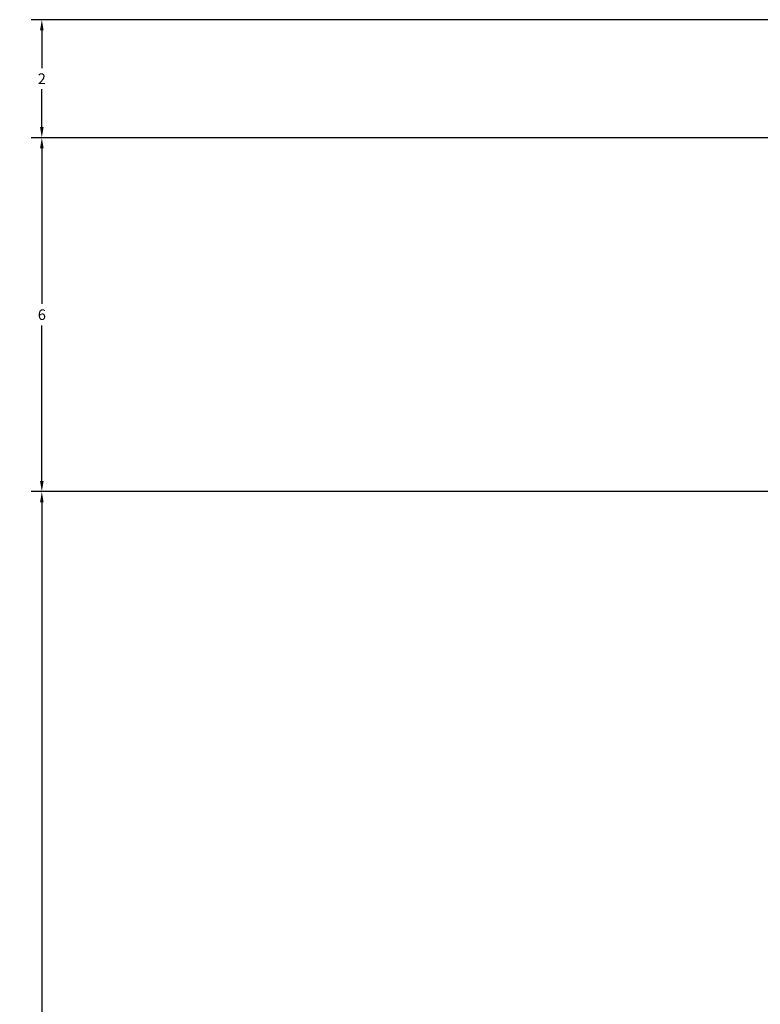
# Model space of a CAD drawing. Units: inches. Extents: x 2812 to 3051, y 1398 to 1659.
# Tile 7 of 65: x 2811.61 to 2824.16, y 1473.34 to 1490.04. Entities that reach past the tile are written whole.
import ezdxf

# ---------------------------------------------------------------- set-up
doc = ezdxf.new("R2010")
doc.units = ezdxf.units.IN
doc.layers.add('A-ANNO-DIMS', color=2, linetype='Continuous', lineweight=18)
doc.styles.get("Standard").update_dxf_attribs({"font": 'arial.ttf'})
doc.dimstyles.get("Standard").update_dxf_attribs({"dimtxt": 0.18, "dimasz": 0.18, "dimexe": 0.18, "dimexo": 0.0625, "dimgap": 0.09, "dimtad": 0, "dimtih": 1, "dimtoh": 1, "dimdec": 4, "dimzin": 0, "dimdsep": 46, "dimtxsty": 'Standard', "dimcen": 0.09, "dimadec": 0, "dimazin": 0, "dimtfac": 1, "dimtdec": 4, "dimtofl": 0, "dimtmove": 0, "dimatfit": 3, "dimfxl": 1, "dimtolj": 1, "dimtzin": 0, "dimarcsym": 0})

# ---------------------------------------------------------------- blocks, each defined once
blk = doc.blocks.new('*D51')
at = {"layer": 'A-ANNO-DIMS', "color": 0, "lineweight": -2, "transparency": 16777216}
for p, q in [((2835.322, 1482.035), (2811.806, 1482.035)), ((2811.986, 1481.855), (2811.986, 1472.351)), ((2811.986, 1462.483), (2811.986, 1471.987)), ((2835.322, 1462.303), (2811.806, 1462.303))]:
    blk.add_line(p, q, dxfattribs=at)
at = {"layer": 'A-ANNO-DIMS', "color": 0, "transparency": 16777216}
for points in [[(2811.956, 1481.855), (2812.016, 1481.855), (2811.986, 1482.035)], [(2811.956, 1462.483), (2812.016, 1462.483), (2811.986, 1462.303)]]:
    blk.add_solid(points, dxfattribs=at)
at = {"layer": 'Defpoints', "color": 0, "transparency": 16777216}
for p in [(2811.986, 1482.035), (2835.385, 1482.035), (2835.385, 1462.303)]:
    blk.add_point(p, dxfattribs=at)
at = {"layer": 'A-ANNO-DIMS', "color": 0, "transparency": 16777216, "insert": (2811.986, 1472.169), "char_height": 0.18, "attachment_point": 5}
blk.add_mtext('\\A1;19.733', dxfattribs=at)
blk = doc.blocks.new('*D52')
at = {"layer": 'A-ANNO-DIMS', "color": 0, "lineweight": -2, "transparency": 16777216}
for p, q in [((2826.322, 1488.035), (2811.806, 1488.035)), ((2811.986, 1487.855), (2811.986, 1485.217)), ((2811.986, 1482.215), (2811.986, 1484.853)), ((2826.322, 1482.035), (2811.806, 1482.035))]:
    blk.add_line(p, q, dxfattribs=at)
at = {"layer": 'A-ANNO-DIMS', "color": 0, "transparency": 16777216}
for points in [[(2811.956, 1487.855), (2812.016, 1487.855), (2811.986, 1488.035)], [(2811.956, 1482.215), (2812.016, 1482.215), (2811.986, 1482.035)]]:
    blk.add_solid(points, dxfattribs=at)
at = {"layer": 'Defpoints', "color": 0, "transparency": 16777216}
for p in [(2811.986, 1488.035), (2826.385, 1488.035), (2826.385, 1482.035)]:
    blk.add_point(p, dxfattribs=at)
at = {"layer": 'A-ANNO-DIMS', "color": 0, "transparency": 16777216, "insert": (2811.986, 1485.035), "char_height": 0.18, "attachment_point": 5}
blk.add_mtext('\\A1;6', dxfattribs=at)
blk = doc.blocks.new('*D53')
at = {"layer": 'A-ANNO-DIMS', "color": 0, "lineweight": -2, "transparency": 16777216}
for p, q in [((2828.322, 1490.035), (2811.806, 1490.035)), ((2811.986, 1489.855), (2811.986, 1489.216)), ((2811.986, 1488.215), (2811.986, 1488.855)), ((2826.322, 1488.035), (2811.806, 1488.035))]:
    blk.add_line(p, q, dxfattribs=at)
at = {"layer": 'A-ANNO-DIMS', "color": 0, "transparency": 16777216}
for points in [[(2811.956, 1489.855), (2812.016, 1489.855), (2811.986, 1490.035)], [(2811.956, 1488.215), (2812.016, 1488.215), (2811.986, 1488.035)]]:
    blk.add_solid(points, dxfattribs=at)
at = {"layer": 'Defpoints', "color": 0, "transparency": 16777216}
for p in [(2811.986, 1490.035), (2828.385, 1490.035), (2826.385, 1488.035)]:
    blk.add_point(p, dxfattribs=at)
at = {"layer": 'A-ANNO-DIMS', "color": 0, "transparency": 16777216, "insert": (2811.986, 1489.035), "char_height": 0.18, "attachment_point": 5}
blk.add_mtext('\\A1;2', dxfattribs=at)

msp = doc.modelspace()

# ---------------------------------------------------------------- dimensions: what is measured, and where the dimension line sits
at = {"layer": 'A-ANNO-DIMS'}
for base, p1, p2, override, picture, middle in [((2811.9855, 1490.0354), (2826.3849, 1488.0354), (2828.3849, 1490.0354), {"dimdec": 0, "dimlfac": 1, "dimrnd": 0, "dimzin": 0, "dimdsep": 46, "dimlunit": 2}, '*D53', (2811.9855, 1489.0354)), ((2811.9855, 1488.0354), (2826.3849, 1482.0354), (2826.3849, 1488.0354), {"dimdec": 0, "dimlfac": 1, "dimrnd": 0, "dimzin": 0, "dimdsep": 46, "dimlunit": 2}, '*D52', (2811.9855, 1485.0354)), ((2811.9855, 1482.0354), (2835.3849, 1462.3026), (2835.3849, 1482.0354), {"dimdec": 3, "dimlfac": 1, "dimrnd": 0, "dimzin": 0, "dimdsep": 46, "dimlunit": 2}, '*D51', (2811.9855, 1472.169))]:
    dim = msp.add_linear_dim(base=base, p1=p1, p2=p2, angle=90, dimstyle='Standard', override=override, dxfattribs=at)
    dim.commit()
    dim.dimension.update_dxf_attribs({"geometry": picture, "text_midpoint": middle})

doc.saveas('drawing.dxf')
